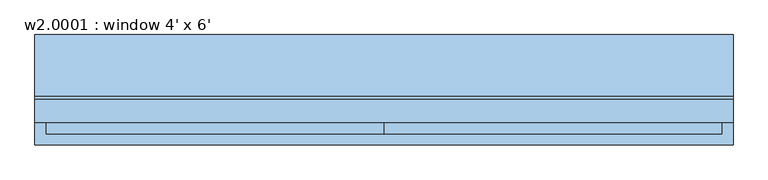
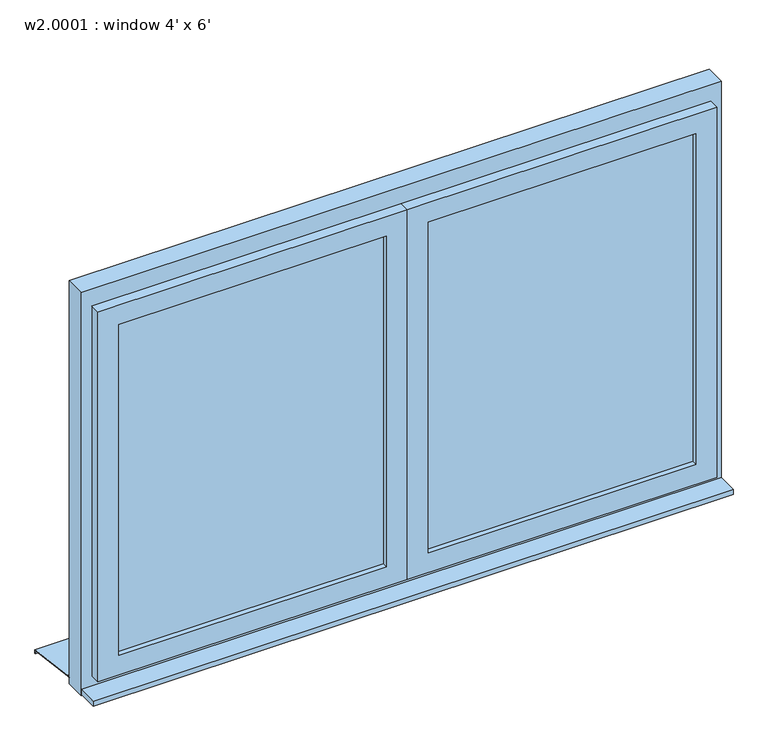
"""IFC4 building model written with IfcOpenShell, lengths in millimetres: window geometry, w2.0001 : window 4' x 6'."""

from ifc_helpers import new_model, si_unit, frame, origin, place, context, project, spatial, polyline, outline, extrude, faceted_brep, source, transform, mapped, element, save


def w2_0001_window_4_x_6_83c3b52c(model_context):
    return source(origin(), model_context, "Body", "SolidModel", [
        extrude(outline(polyline([(-15.6778457, 1020.0), (144.3, 1000.0), (144.3, 990.0), (142.3, 990.0), (142.3, 998.3604634), (-15.8759277, 1018.0), (-25.7, 1018.0), (-25.7, 1020.0), (-15.6778457, 1020.0)])), frame((-914.4, 0.0, 0.0), z_axis=(1.0, 0.0, 0.0), x_axis=(0.0, 1.0, 0.0)), (0.0, 0.0, 1.0), 1828.8),
        extrude(outline(polyline([(-914.4, -144.3), (-914.4, -85.7), (914.4, -85.7), (914.4, -144.3), (-914.4, -144.3)])), frame((0.0, 0.0, 1005.0), z_axis=(0.0, 0.0, 1.0), x_axis=(1.0, 0.0, 0.0)), (0.0, 0.0, 1.0), 15.0),
        extrude(outline(polyline([(60.0, -70.7), (824.4, -70.7), (824.4, -100.7), (60.0, -100.7), (60.0, -70.7)])), frame((0.0, 0.0, 1110.0), z_axis=(0.0, 0.0, 1.0), x_axis=(1.0, 0.0, 0.0)), (0.0, 0.0, 1.0), 999.2),
        extrude(outline(polyline([(-824.4, -70.7), (-60.0, -70.7), (-60.0, -100.7), (-824.4, -100.7), (-824.4, -70.7)])), frame((0.0, 0.0, 1110.0), z_axis=(0.0, 0.0, 1.0), x_axis=(1.0, 0.0, 0.0)), (0.0, 0.0, 1.0), 999.2),
        extrude(outline(polyline([(2219.2, -914.4), (1000.0, -914.4), (1000.0, 914.4), (2219.2, 914.4), (2219.2, -914.4)]), holes=[polyline([(2139.2, -854.4), (2139.2, 854.4), (1080.0, 854.4), (1080.0, -854.4), (2139.2, -854.4)])]), frame((0.0, -85.7, 0.0), z_axis=(0.0, 1.0, 0.0), x_axis=(0.0, 0.0, 1.0)), (0.0, 0.0, 1.0), 60.0),
        extrude(outline(polyline([(30.0, -85.7), (-30.0, -85.7), (-30.0, -25.7), (30.0, -25.7), (30.0, -85.7)])), frame((0.0, 0.0, 1080.0), z_axis=(0.0, 0.0, 1.0), x_axis=(1.0, 0.0, 0.0)), (0.0, 0.0, 1.0), 1059.2),
        faceted_brep([(30.0, -85.7, 1080.0), (30.0, -55.7, 1080.0), (854.4, -55.7, 1080.0), (854.4, -85.7, 1080.0), (854.4, -55.7, 2139.2), (854.4, -85.7, 2139.2), (30.0, -55.7, 2139.2), (824.4, -55.7, 2109.2), (60.0, -55.7, 2109.2), (60.0, -55.7, 1110.0), (824.4, -55.7, 1110.0), (884.4, -85.7, 1050.0), (0.0, -85.7, 1050.0), (0.0, -85.7, 2169.2), (884.4, -85.7, 2169.2), (30.0, -85.7, 2139.2), (0.0, -115.7, 1050.0), (884.4, -115.7, 1050.0), (884.4, -115.7, 2169.2), (0.0, -115.7, 2169.2), (824.4, -115.7, 1110.0), (60.0, -115.7, 1110.0), (60.0, -115.7, 2109.2), (824.4, -115.7, 2109.2)], [[[0, 1, 2, 3]], [[3, 2, 4, 5]], [[2, 1, 6, 4], [7, 8, 9, 10]], [[11, 12, 13, 14], [5, 15, 0, 3]], [[16, 12, 11, 17]], [[17, 11, 14, 18]], [[18, 19, 16, 17], [20, 21, 22, 23]], [[9, 21, 20, 10]], [[10, 20, 23, 7]], [[15, 6, 1, 0]], [[19, 13, 12, 16]], [[8, 22, 21, 9]], [[5, 4, 6, 15]], [[18, 14, 13, 19]], [[7, 23, 22, 8]]]),
        faceted_brep([(-854.4, -85.7, 1080.0), (-854.4, -55.7, 1080.0), (-30.0, -55.7, 1080.0), (-30.0, -85.7, 1080.0), (-30.0, -55.7, 2139.2), (-30.0, -85.7, 2139.2), (-854.4, -55.7, 2139.2), (-60.0, -55.7, 2109.2), (-824.4, -55.7, 2109.2), (-824.4, -55.7, 1110.0), (-60.0, -55.7, 1110.0), (0.0, -85.7, 1050.0), (-884.4, -85.7, 1050.0), (-884.4, -85.7, 2169.2), (0.0, -85.7, 2169.2), (-854.4, -85.7, 2139.2), (-884.4, -115.7, 1050.0), (0.0, -115.7, 1050.0), (0.0, -115.7, 2169.2), (-884.4, -115.7, 2169.2), (-60.0, -115.7, 1110.0), (-824.4, -115.7, 1110.0), (-824.4, -115.7, 2109.2), (-60.0, -115.7, 2109.2)], [[[0, 1, 2, 3]], [[3, 2, 4, 5]], [[2, 1, 6, 4], [7, 8, 9, 10]], [[11, 12, 13, 14], [5, 15, 0, 3]], [[16, 12, 11, 17]], [[17, 11, 14, 18]], [[18, 19, 16, 17], [20, 21, 22, 23]], [[9, 21, 20, 10]], [[10, 20, 23, 7]], [[15, 6, 1, 0]], [[19, 13, 12, 16]], [[8, 22, 21, 9]], [[5, 4, 6, 15]], [[18, 14, 13, 19]], [[7, 23, 22, 8]]]),
    ])


if __name__ == "__main__":
    model = new_model("IFC4")
    model_context = context("Model", 3, world=origin())
    ifc_project = project(units=[si_unit("LENGTHUNIT", "METRE", prefix="MILLI")], contexts=[model_context])
    site = spatial("IfcSite", under=ifc_project)
    building = spatial("IfcBuilding", under=site)
    placement = place(None, origin())
    w2_0001_window_4_x_6_shape = w2_0001_window_4_x_6_83c3b52c(model_context)
    element("IfcWindow", 1, ObjectType="w2.0001 : window 4' x 6'", at=placement, inside=building, context=model_context, shape_type="MappedRepresentation", body=[
        mapped(w2_0001_window_4_x_6_shape, transform((0.0, 0.0, 0.0), x_axis=(1.0, 0.0, 0.0), y_axis=(0.0, 1.0, 0.0), z_axis=(0.0, 0.0, 1.0))),
    ])
    save(model, "model.ifc")

# Revit data of these elements
# Type "w2.0001 : window 4' x 6'"
#   Type Mark = "22"
#   Operation = "DoublePanelVertical"
#   Keynote = "16.05.01"
#   Analytic Construction = "<None>"
#   Rough Width = 6' - 0"
#   Rough Height = 4' - 0"
#   Rahmentiefe = 0' - 2.3622"
#   Rahmenhöhe unten = 0' - 3.14961"
#   Rahmehöhe oben = 0' - 3.14961"
#   Rahmenbreite = 0' - 2.3622"
#   Height = 4' - 0"
#   Flügeltiefe = 0' - 2.3622"
#   Flügelbreite = 0' - 2.3622"
#   Einbautiefe (von außen) [instance default] = 0' - 5.51181"
#   Width = 6' - 0"
#   Kippflügel [instance default] = yes
#   Drehflügel im Grundriß darstellen [instance default] = no
#   Drehflügel [instance default] = yes
#   Define Thermal Properties by = 1
#   Rahmen [instance default] = none
#   Glas [instance default] = none
#   Flügel [instance default] = none
#   Fensterbank aussen [instance default] = none
#   Fensterbank innen [instance default] = none
#   Wall Closure = (empty or 0)
# Element 1 (IfcWindow, "w2.0001 : window 4' x 6'")
#   Materials on its faces: "Fenster - Kunststoff", "Fenster - Kunststoff weiss", "Glass", "Fenster - Holz"
# Materials
#   "Fenster - Kunststoff": colour RGB 249 249 249, transparency 0
#   "Fenster - Kunststoff weiss": colour RGB 249 249 249, transparency 0
#   "Glass": class "Glass", colour RGB 0 128 192, transparency 0.75, Description = "Soda Lime Glass", Cost = 0
#   "Fenster - Holz": colour RGB 216 135 75, transparency 0
